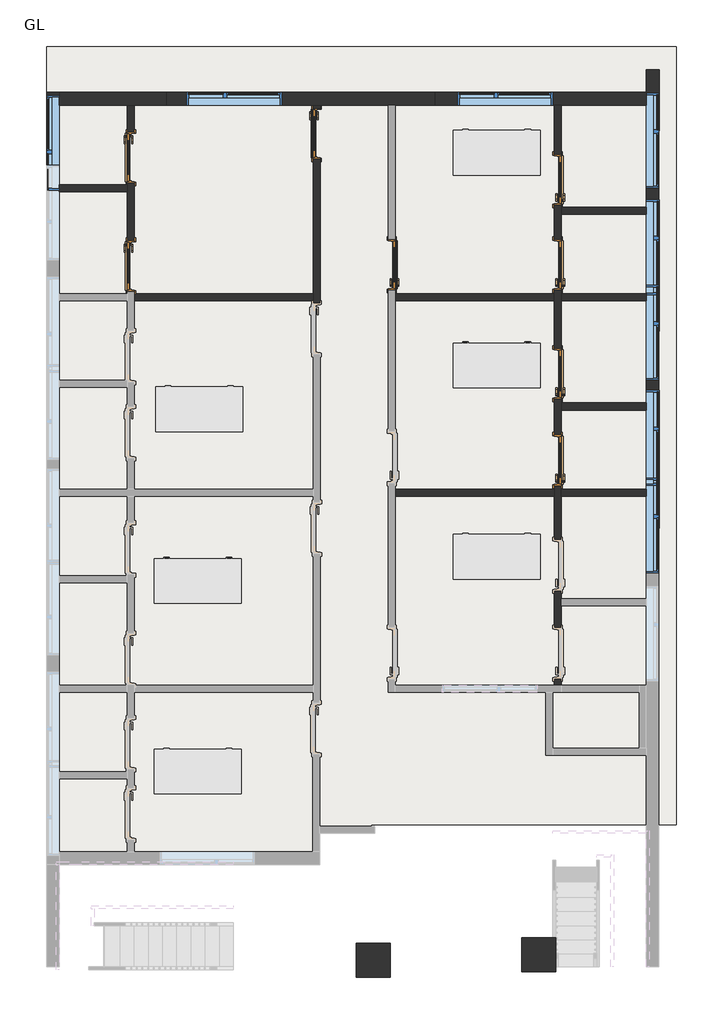
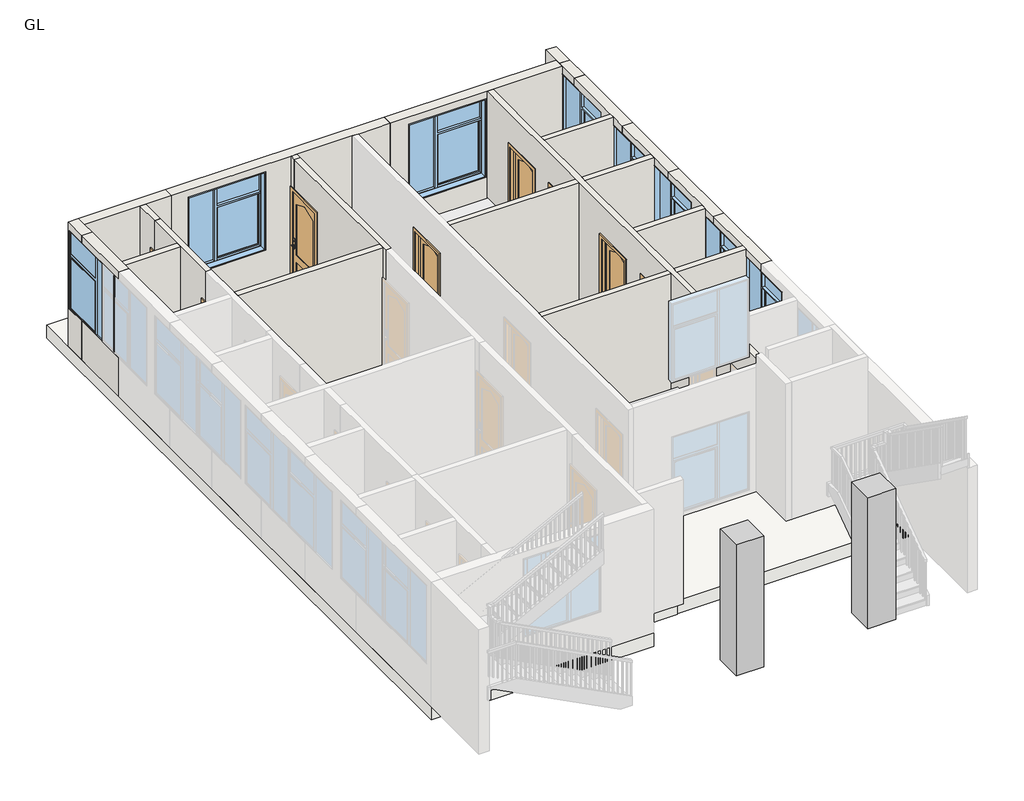
# One storey, part 2 of 4: 24 walls, 8 doors, 8 windows, 2 columns, 1 slab.
"""IFC4 building model written with IfcOpenShell, lengths in millimetres."""

from ifc_helpers import new_model, si_unit, frame, origin, origin_with_axes, place, context, project, spatial, polyline, outline, extrude, faceted_brep, transform, mapped, element, save
from components import column_c091e905, door_346b4a94, m_window_casement_double_sidelight_1702_x_1829mm_c8b42c7f

model = new_model("IFC4")

# Units and contexts
model_context = context("Model", 3, world=origin())
ifc_project = project(units=[si_unit("LENGTHUNIT", "METRE", prefix="MILLI")], contexts=[model_context])

# Site, building, storey
site = spatial("IfcSite", under=ifc_project)
building = spatial("IfcBuilding", under=site)
storey = spatial("IfcBuildingStorey", under=building, Name="GL", Elevation=0.0)

# Columns
placement = place(None, origin())
element("IfcColumn", 1, ObjectType="Rectangular Column : 24\" x 24\"", at=placement, inside=storey, context=model_context, shape_type="SweptSolid", body=[
    extrude(outline(polyline([(2657.4891134, -7132.8082131), (2657.4891134, -7742.4082131), (2047.8891134, -7742.4082131), (2047.8891134, -7132.8082131), (2657.4891134, -7132.8082131)])), origin_with_axes(), (0.0, 0.0, 1.0), 3048.0),
])
column_shape = column_c091e905(model_context)
element("IfcColumn", 2, ObjectType="Rectangular Column : 24\" x 24\"", at=placement, inside=storey, context=model_context, shape_type="MappedRepresentation", body=[
    mapped(column_shape, transform((-606.4108866, -7539.2082131, 0.0), x_axis=(1.0, 0.0, 0.0), y_axis=(0.0, 1.0, 0.0), z_axis=(0.0, 0.0, 1.0))),
])

# Doors
door_shape = door_346b4a94(model_context)
element("IfcDoor", 3, ObjectType="2'10\"X7'", at=placement, inside=storey, context=model_context, shape_type="MappedRepresentation", body=[
    mapped(door_shape, transform((2698.7641134, 6449.4399728, 0.0), x_axis=(0.0, -1.0, 0.0), y_axis=(1.0, 0.0, 0.0), z_axis=(0.0, 0.0, 1.0))),
])
element("IfcDoor", 4, ObjectType="2'10\"X7'", at=placement, inside=storey, context=model_context, shape_type="MappedRepresentation", body=[
    mapped(door_shape, transform((2698.7641134, 4925.4399728, 0.0), x_axis=(0.0, -1.0, 0.0), y_axis=(1.0, 0.0, 0.0), z_axis=(0.0, 0.0, 1.0))),
])
element("IfcDoor", 5, ObjectType="2'10\"X7'", at=placement, inside=storey, context=model_context, shape_type="MappedRepresentation", body=[
    mapped(door_shape, transform((2698.7641134, 2969.6399728, 0.0), x_axis=(0.0, -1.0, 0.0), y_axis=(1.0, 0.0, 0.0), z_axis=(0.0, 0.0, 1.0))),
])
element("IfcDoor", 6, ObjectType="2'10\"X7'", at=placement, inside=storey, context=model_context, shape_type="MappedRepresentation", body=[
    mapped(door_shape, transform((2698.7641134, 1420.2399728, 0.0), x_axis=(0.0, -1.0, 0.0), y_axis=(1.0, 0.0, 0.0), z_axis=(0.0, 0.0, 1.0))),
])
element("IfcDoor", 7, ObjectType="2'10\"X7'", at=placement, inside=storey, context=model_context, shape_type="MappedRepresentation", body=[
    mapped(door_shape, transform((-273.0358866, 4925.4399728, 0.0), x_axis=(0.0, -1.0, 0.0), y_axis=(1.0, 0.0, 0.0), z_axis=(0.0, 0.0, 1.0))),
])
element("IfcDoor", 8, ObjectType="2'10\"X7'", at=placement, inside=storey, context=model_context, shape_type="MappedRepresentation", body=[
    mapped(door_shape, transform((-4952.9858866, 4900.320652, 0.0), x_axis=(0.0, 1.0, 0.0), y_axis=(-1.0, 0.0, 0.0), z_axis=(0.0, 0.0, 1.0))),
])
element("IfcDoor", 9, ObjectType="2'10\"X7'", at=placement, inside=storey, context=model_context, shape_type="MappedRepresentation", body=[
    mapped(door_shape, transform((-4952.9858866, 6843.9929737, 0.0), x_axis=(0.0, 1.0, 0.0), y_axis=(-1.0, 0.0, 0.0), z_axis=(0.0, 0.0, 1.0))),
])
element("IfcDoor", 10, ObjectType="2'10\"X7'", at=placement, inside=storey, context=model_context, shape_type="MappedRepresentation", body=[
    mapped(door_shape, transform((-1625.5858866, 7274.3310623, 0.0), x_axis=(0.0, 1.0, 0.0), y_axis=(-1.0, 0.0, 0.0), z_axis=(0.0, 0.0, 1.0))),
])

# Slab
element("IfcSlab", 11, ObjectType="Generic - 12\"", at=placement, inside=storey, context=model_context, shape_type="SweptSolid", body=[
    extrude(outline(polyline([(4816.4891134, 8833.6177996), (4816.4891134, -5110.9822004), (-644.5108866, -5110.9822004), (-644.5108866, -5136.3822004), (-1562.4669858, -5136.3822004), (-1562.4669858, -5824.7082131), (-6461.1108866, -5824.7082131), (-6461.1108866, 8833.6177996), (4816.4891134, 8833.6177996)])), frame((0.0, 0.0, -304.8), z_axis=(0.0, 0.0, 1.0), x_axis=(1.0, 0.0, 0.0)), (0.0, 0.0, 1.0), 304.8),
])

# Walls
element("IfcWall", 12, ObjectType="Generic - 4.5\"", at=placement, inside=storey, context=model_context, shape_type="SweptSolid", body=[
    extrude(outline(polyline([(7782.9399728, 2895.6), (7782.9399728, 0.0), (7300.7929737, 0.0), (7300.7929737, 2158.6), (7224.9929737, 2158.6), (7224.9929737, 2895.6), (7782.9399728, 2895.6)])), frame((-5013.3108866, 0.0, 0.0), z_axis=(1.0, 0.0, 0.0), x_axis=(0.0, 1.0, 0.0)), (0.0, 0.0, 1.0), 127.0),
])
element("IfcWall", 13, ObjectType="Generic - 4.5\"", at=placement, inside=storey, context=model_context, shape_type="Brep", body=[
    faceted_brep([(-5013.3108866, 5281.320652, 2158.6), (-5013.3108866, 5281.320652, 2895.6), (-5013.3108866, 6233.5399728, 2895.6), (-5013.3108866, 6360.5399728, 2895.6), (-5013.3108866, 7224.9929737, 2895.6), (-5013.3108866, 7224.9929737, 2158.6), (-5013.3108866, 6387.1929737, 2158.6), (-5013.3108866, 6387.1929737, 0.0), (-5013.3108866, 6360.5399728, 0.0), (-5013.3108866, 6233.5399728, 0.0), (-5013.3108866, 5357.120652, 0.0), (-5013.3108866, 5357.120652, 2158.6), (-4886.3108866, 5281.320652, 2895.6), (-4886.3108866, 5281.320652, 2158.6), (-4886.3108866, 5357.120652, 2158.6), (-4886.3108866, 5357.120652, 0.0), (-4886.3108866, 6387.1929737, 0.0), (-4886.3108866, 6387.1929737, 2158.6), (-4886.3108866, 7224.9929737, 2158.6), (-4886.3108866, 7224.9929737, 2895.6)], [[[0, 1, 2, 3, 4, 5, 6, 7, 8, 9, 10, 11]], [[12, 13, 14, 15, 16, 17, 18, 19]], [[15, 10, 9, 8, 7, 16]], [[1, 0, 13, 12]], [[4, 19, 18, 5]], [[14, 11, 10, 15]], [[11, 14, 13, 0]], [[17, 6, 5, 18]], [[6, 17, 16, 7]], [[4, 3, 2, 1, 12, 19]]]),
])
element("IfcWall", 14, ObjectType="Generic - 4.5\"", at=placement, inside=storey, context=model_context, shape_type="SweptSolid", body=[
    extrude(outline(polyline([(-5013.3108866, 6233.5399728), (-6232.5508078, 6233.5399728), (-6232.5508078, 6360.5399728), (-5013.3108866, 6360.5399728), (-5013.3108866, 6233.5399728)])), origin_with_axes(), (0.0, 0.0, 1.0), 2895.6),
])
element("IfcWall", 15, ObjectType="Generic - 4.5\"", at=placement, inside=storey, context=model_context, shape_type="SweptSolid", body=[
    extrude(outline(polyline([(-1685.9108866, 4277.7399728), (-4886.3108866, 4277.7399728), (-4886.3108866, 4404.7399728), (-1685.9108866, 4404.7399728), (-1685.9108866, 4277.7399728)])), origin_with_axes(), (0.0, 0.0, 1.0), 2895.6),
])
element("IfcWall", 16, ObjectType="Generic - 4.5\"", at=placement, inside=storey, context=model_context, shape_type="SweptSolid", body=[
    extrude(outline(polyline([(7782.9399728, 2895.6), (7782.9399728, 0.0), (7731.1310623, 0.0), (7731.1310623, 2158.6), (7655.3310623, 2158.6), (7655.3310623, 2895.6), (7782.9399728, 2895.6)])), frame((-1685.9108866, 0.0, 0.0), z_axis=(1.0, 0.0, 0.0), x_axis=(0.0, 1.0, 0.0)), (0.0, 0.0, 1.0), 127.0),
])
element("IfcWall", 17, ObjectType="Generic - 4.5\"", at=placement, inside=storey, context=model_context, shape_type="Brep", body=[
    faceted_brep([(-1685.9108866, 4182.2008884, 2158.6), (-1685.9108866, 4182.2008884, 2895.6), (-1685.9108866, 4277.7399728, 2895.6), (-1685.9108866, 4404.7399728, 2895.6), (-1685.9108866, 7655.3310623, 2895.6), (-1685.9108866, 7655.3310623, 2158.6), (-1685.9108866, 6817.5310623, 2158.6), (-1685.9108866, 6817.5310623, 0.0), (-1685.9108866, 4404.7399728, 0.0), (-1685.9108866, 4277.7399728, 0.0), (-1685.9108866, 4232.6008884, 0.0), (-1685.9108866, 4232.6008884, 2158.6), (-1558.9108866, 4182.2008884, 2895.6), (-1558.9108866, 4182.2008884, 2158.6), (-1558.9108866, 4232.6008884, 2158.6), (-1558.9108866, 4232.6008884, 0.0), (-1558.9108866, 6817.5310623, 0.0), (-1558.9108866, 6817.5310623, 2158.6), (-1558.9108866, 7655.3310623, 2158.6), (-1558.9108866, 7655.3310623, 2895.6), (-1685.4871817, 4182.2008884, 2158.6), (-1685.4871817, 4182.2008884, 2895.6)], [[[0, 1, 2, 3, 4, 5, 6, 7, 8, 9, 10, 11]], [[12, 13, 14, 15, 16, 17, 18, 19]], [[15, 10, 9, 8, 7, 16]], [[1, 0, 20, 13, 12, 21]], [[4, 19, 18, 5]], [[14, 11, 10, 15]], [[11, 14, 13, 20, 0]], [[17, 6, 5, 18]], [[6, 17, 16, 7]], [[4, 3, 2, 1, 21, 12, 19]]]),
])
element("IfcWall", 18, ObjectType="Generic - 4.5\"", at=placement, inside=storey, context=model_context, shape_type="Brep", body=[
    faceted_brep([(2632.0891134, 7782.9399728, 2895.6), (2632.0891134, 7782.9399728, 0.0), (2632.0891134, 6906.2399728, 0.0), (2632.0891134, 6906.2399728, 2158.6), (2632.0891134, 5992.6399728, 2158.6), (2632.0891134, 5992.6399728, 0.0), (2632.0891134, 5382.2399728, 0.0), (2632.0891134, 5382.2399728, 2158.6), (2632.0891134, 4468.6399728, 2158.6), (2632.0891134, 4468.6399728, 0.0), (2632.0891134, 4404.7399728, 0.0), (2632.0891134, 4277.7399728, 0.0), (2632.0891134, 3426.4399728, 0.0), (2632.0891134, 3426.4399728, 2158.6), (2632.0891134, 2512.8399728, 2158.6), (2632.0891134, 2512.8399728, 0.0), (2632.0891134, 1877.0399728, 0.0), (2632.0891134, 1877.0399728, 2158.6), (2632.0891134, 963.4399728, 2158.6), (2632.0891134, 963.4399728, 0.0), (2632.0891134, 899.5399728, 0.0), (2632.0891134, 772.5399728, 0.0), (2632.0891134, -2.5600272, 0.0), (2632.0891134, -2.5600272, 2158.6), (2632.0891134, -916.1600272, 2158.6), (2632.0891134, -916.1600272, 0.0), (2632.0891134, -1577.3600272, 0.0), (2632.0891134, -1577.3600272, 2158.6), (2632.0891134, -2490.9600272, 2158.6), (2632.0891134, -2490.9600272, 0.0), (2632.0891134, -2605.6600272, 0.0), (2632.0891134, -2605.6600272, 2895.6), (2632.0891134, 772.5399728, 2895.6), (2632.0891134, 899.5399728, 2895.6), (2632.0891134, 4277.7399728, 2895.6), (2632.0891134, 4404.7399728, 2895.6), (2759.0891134, 7782.9399728, 0.0), (2759.0891134, 7782.9399728, 2895.6), (2759.0891134, 5954.1399728, 2895.6), (2759.0891134, 5827.1399728, 2895.6), (2759.0891134, 4404.7399728, 2895.6), (2759.0891134, 4277.7399728, 2895.6), (2759.0891134, 2448.9399728, 2895.6), (2759.0891134, 2321.9399728, 2895.6), (2759.0891134, 899.5399728, 2895.6), (2759.0891134, 772.5399728, 2895.6), (2759.0891134, -1056.2600272, 2895.6), (2759.0891134, -1183.2600272, 2895.6), (2759.0891134, -2605.6600272, 2895.6), (2759.0891134, -2605.6600272, 0.0), (2759.0891134, -2490.9600272, 0.0), (2759.0891134, -2490.9600272, 2158.6), (2759.0891134, -1577.3600272, 2158.6), (2759.0891134, -1577.3600272, 0.0), (2759.0891134, -1183.2600272, 0.0), (2759.0891134, -1056.2600272, 0.0), (2759.0891134, -916.1600272, 0.0), (2759.0891134, -916.1600272, 2158.6), (2759.0891134, -2.5600272, 2158.6), (2759.0891134, -2.5600272, 0.0), (2759.0891134, 772.5399728, 0.0), (2759.0891134, 899.5399728, 0.0), (2759.0891134, 963.4399728, 0.0), (2759.0891134, 963.4399728, 2158.6), (2759.0891134, 1877.0399728, 2158.6), (2759.0891134, 1877.0399728, 0.0), (2759.0891134, 2321.9399728, 0.0), (2759.0891134, 2448.9399728, 0.0), (2759.0891134, 2512.8399728, 0.0), (2759.0891134, 2512.8399728, 2158.6), (2759.0891134, 3426.4399728, 2158.6), (2759.0891134, 3426.4399728, 0.0), (2759.0891134, 4277.7399728, 0.0), (2759.0891134, 4404.7399728, 0.0), (2759.0891134, 4468.6399728, 0.0), (2759.0891134, 4468.6399728, 2158.6), (2759.0891134, 5382.2399728, 2158.6), (2759.0891134, 5382.2399728, 0.0), (2759.0891134, 5827.1399728, 0.0), (2759.0891134, 5954.1399728, 0.0), (2759.0891134, 5992.6399728, 0.0), (2759.0891134, 5992.6399728, 2158.6), (2759.0891134, 6906.2399728, 2158.6), (2759.0891134, 6906.2399728, 0.0)], [[[0, 1, 2, 3, 4, 5, 6, 7, 8, 9, 10, 11, 12, 13, 14, 15, 16, 17, 18, 19, 20, 21, 22, 23, 24, 25, 26, 27, 28, 29, 30, 31, 32, 33, 34, 35]], [[36, 37, 38, 39, 40, 41, 42, 43, 44, 45, 46, 47, 48, 49, 50, 51, 52, 53, 54, 55, 56, 57, 58, 59, 60, 61, 62, 63, 64, 65, 66, 67, 68, 69, 70, 71, 72, 73, 74, 75, 76, 77, 78, 79, 80, 81, 82, 83]], [[1, 36, 83, 2]], [[5, 80, 79, 78, 77, 6]], [[9, 74, 73, 72, 71, 12, 11, 10]], [[15, 68, 67, 66, 65, 16]], [[19, 62, 61, 60, 59, 22, 21, 20]], [[25, 56, 55, 54, 53, 26]], [[49, 30, 29, 50]], [[1, 0, 37, 36]], [[4, 81, 80, 5]], [[81, 4, 3, 82]], [[82, 3, 2, 83]], [[9, 8, 75, 74]], [[8, 7, 76, 75]], [[7, 6, 77, 76]], [[14, 69, 68, 15]], [[69, 14, 13, 70]], [[70, 13, 12, 71]], [[18, 63, 62, 19]], [[63, 18, 17, 64]], [[64, 17, 16, 65]], [[24, 57, 56, 25]], [[57, 24, 23, 58]], [[58, 23, 22, 59]], [[28, 51, 50, 29]], [[51, 28, 27, 52]], [[52, 27, 26, 53]], [[0, 35, 34, 33, 32, 31, 48, 47, 46, 45, 44, 43, 42, 41, 40, 39, 38, 37]], [[31, 30, 49, 48]]]),
])
element("IfcWall", 19, ObjectType="Generic - 4.5\"", at=placement, inside=storey, context=model_context, shape_type="SweptSolid", body=[
    extrude(outline(polyline([(2632.0891134, 4277.7399728), (-212.7108866, 4277.7399728), (-212.7108866, 4404.7399728), (2632.0891134, 4404.7399728), (2632.0891134, 4277.7399728)])), origin_with_axes(), (0.0, 0.0, 1.0), 2895.6),
])
element("IfcWall", 20, ObjectType="Generic - 4.5\"", at=placement, inside=storey, context=model_context, shape_type="SweptSolid", body=[
    extrude(outline(polyline([(2632.0891134, 772.5399728), (-212.7108866, 772.5399728), (-212.7108866, 899.5399728), (2632.0891134, 899.5399728), (2632.0891134, 772.5399728)])), origin_with_axes(), (0.0, 0.0, 1.0), 2895.6),
])
element("IfcWall", 21, ObjectType="Generic - 4.5\"", at=placement, inside=storey, context=model_context, shape_type="SweptSolid", body=[
    extrude(outline(polyline([(4281.587404, 5827.1399728), (2759.0891134, 5827.1399728), (2759.0891134, 5954.1399728), (4281.587404, 5954.1399728), (4281.587404, 5827.1399728)])), origin_with_axes(), (0.0, 0.0, 1.0), 2895.6),
])
element("IfcWall", 22, ObjectType="Generic - 4.5\"", at=placement, inside=storey, context=model_context, shape_type="SweptSolid", body=[
    extrude(outline(polyline([(4283.9989713, 4277.7399728), (2759.0891134, 4277.7399728), (2759.0891134, 4404.7399728), (4283.9989713, 4404.7399728), (4283.9989713, 4277.7399728)])), origin_with_axes(), (0.0, 0.0, 1.0), 2895.6),
])
element("IfcWall", 23, ObjectType="Generic - 4.5\"", at=placement, inside=storey, context=model_context, shape_type="SweptSolid", body=[
    extrude(outline(polyline([(4281.0767915, 2321.9399728), (2759.0891134, 2321.9399728), (2759.0891134, 2448.9399728), (4281.0767915, 2448.9399728), (4281.0767915, 2321.9399728)])), origin_with_axes(), (0.0, 0.0, 1.0), 2895.6),
])
element("IfcWall", 24, ObjectType="Generic - 4.5\"", at=placement, inside=storey, context=model_context, shape_type="SweptSolid", body=[
    extrude(outline(polyline([(4283.0918814, 772.5399728), (2759.0891134, 772.5399728), (2759.0891134, 899.5399728), (4283.0918814, 899.5399728), (4283.0918814, 772.5399728)])), origin_with_axes(), (0.0, 0.0, 1.0), 2895.6),
])
element("IfcWall", 25, ObjectType="Generic - 9\"", at=placement, inside=storey, context=model_context, shape_type="Brep", body=[
    faceted_brep([(-6232.5108866, 7782.9399728, 0.0), (-5013.3108866, 7782.9399728, 0.0), (-4886.3108866, 7782.9399728, 0.0), (-4318.2603585, 7782.9399728, 0.0), (-4318.2603585, 7782.9399728, 2895.6), (-4886.3108866, 7782.9399728, 2895.6), (-5013.3108866, 7782.9399728, 2895.6), (-6232.5108866, 7782.9399728, 2895.6), (-6232.5108866, 8011.5399728, 0.0), (-6232.5108866, 8011.5399728, 2895.6), (-4318.2603585, 8011.5399728, 2895.6), (-4318.2603585, 8011.5399728, 0.0)], [[[0, 1, 2, 3, 4, 5, 6, 7]], [[8, 9, 10, 11]], [[3, 2, 1, 0, 8, 11]], [[4, 3, 11, 10]], [[0, 7, 9, 8]], [[7, 6, 5, 4, 10, 9]]]),
])
element("IfcWall", 26, ObjectType="Generic - 9\"", at=placement, inside=storey, context=model_context, shape_type="Brep", body=[
    faceted_brep([(-4318.2603585, 7782.9399728, 0.0), (-1685.9108866, 7782.9399728, 0.0), (-1558.9108866, 7782.9399728, 0.0), (-339.7108866, 7782.9399728, 0.0), (-212.7108866, 7782.9399728, 0.0), (496.3553976, 7782.9399728, 0.0), (496.3553976, 7782.9399728, 2895.6), (-212.7108866, 7782.9399728, 2895.6), (-339.7108866, 7782.9399728, 2895.6), (-1558.9108866, 7782.9399728, 2895.6), (-1685.9108866, 7782.9399728, 2895.6), (-4318.2603585, 7782.9399728, 2895.6), (-2248.1603585, 7782.9399728, 2728.8), (-2248.1603585, 7782.9399728, 900.0), (-3949.9603585, 7782.9399728, 900.0), (-3949.9603585, 7782.9399728, 2728.8), (-4318.2603585, 8011.5399728, 0.0), (-4318.2603585, 8011.5399728, 2895.6), (496.3553976, 8011.5399728, 2895.6), (496.3553976, 8011.5399728, 0.0), (-2248.1603585, 8011.5399728, 2728.8), (-3949.9603585, 8011.5399728, 2728.8), (-3949.9603585, 8011.5399728, 900.0), (-2248.1603585, 8011.5399728, 900.0)], [[[0, 1, 2, 3, 4, 5, 6, 7, 8, 9, 10, 11], [12, 13, 14, 15]], [[16, 17, 18, 19], [20, 21, 22, 23]], [[5, 4, 3, 2, 1, 0, 16, 19]], [[6, 5, 19, 18]], [[0, 11, 17, 16]], [[13, 12, 20, 23]], [[14, 13, 23, 22]], [[15, 14, 22, 21]], [[12, 15, 21, 20]], [[11, 10, 9, 8, 7, 6, 18, 17]]]),
])
element("IfcWall", 27, ObjectType="Generic - 9\"", at=placement, inside=storey, context=model_context, shape_type="Brep", body=[
    faceted_brep([(496.3553976, 7782.9399728, 0.0), (2632.0891134, 7782.9399728, 0.0), (2759.0891134, 7782.9399728, 0.0), (4283.0891134, 7782.9399728, 0.0), (4283.0891134, 7782.9399728, 2895.6), (2759.0891134, 7782.9399728, 2895.6), (2632.0891134, 7782.9399728, 2895.6), (496.3553976, 7782.9399728, 2895.6), (2606.6891134, 7782.9399728, 2728.8), (2606.6891134, 7782.9399728, 900.0), (904.8891134, 7782.9399728, 900.0), (904.8891134, 7782.9399728, 2728.8), (496.3553976, 8011.5399728, 0.0), (496.3553976, 8011.5399728, 2895.6), (4283.0891134, 8011.5399728, 2895.6), (4283.0891134, 8011.5399728, 0.0), (2606.6891134, 8011.5399728, 2728.8), (904.8891134, 8011.5399728, 2728.8), (904.8891134, 8011.5399728, 900.0), (2606.6891134, 8011.5399728, 900.0), (4283.0891134, 7897.2399728, 0.0), (4283.0891134, 7897.2399728, 2895.6)], [[[0, 1, 2, 3, 4, 5, 6, 7], [8, 9, 10, 11]], [[12, 13, 14, 15], [16, 17, 18, 19]], [[3, 2, 1, 0, 12, 15, 20]], [[0, 7, 13, 12]], [[9, 8, 16, 19]], [[10, 9, 19, 18]], [[11, 10, 18, 17]], [[8, 11, 17, 16]], [[4, 3, 20, 15, 14, 21]], [[7, 6, 5, 4, 21, 14, 13]]]),
])
element("IfcWall", 28, ObjectType="Generic - 9\"", at=placement, inside=storey, context=model_context, shape_type="Brep", body=[
    faceted_brep([(4283.0891134, 7897.2399728, 0.0), (4283.0891134, 7782.9399728, 0.0), (4283.0891134, 7325.7399728, 0.0), (4283.0891134, 7325.7399728, 900.0), (4283.0891134, 7897.2399728, 900.0), (4511.6891134, 7325.7399728, 0.0), (4511.6891134, 7897.2399728, 0.0), (4511.6891134, 7897.2399728, 900.0), (4511.6891134, 7325.7399728, 900.0), (4510.187404, 7325.7399728, 0.0), (4510.187404, 7325.7399728, 900.0)], [[[0, 1, 2, 3, 4]], [[5, 6, 7, 8]], [[2, 1, 0, 6, 5, 9]], [[2, 9, 5, 8, 10, 3]], [[6, 0, 4, 7]], [[4, 3, 10, 8, 7]]]),
    faceted_brep([(4283.0891134, 7325.7399728, 2895.6), (4283.0891134, 7782.9399728, 2895.6), (4283.0891134, 7897.2399728, 2895.6), (4283.0891134, 7897.2399728, 2728.8), (4283.0891134, 7325.7399728, 2728.8), (4511.6891134, 7897.2399728, 2895.6), (4511.6891134, 7325.7399728, 2895.6), (4511.6891134, 7325.7399728, 2728.8), (4511.6891134, 7897.2399728, 2728.8), (4510.187404, 7325.7399728, 2895.6), (4510.187404, 7325.7399728, 2728.8)], [[[0, 1, 2, 3, 4]], [[5, 6, 7, 8]], [[6, 9, 0, 4, 10, 7]], [[2, 5, 8, 3]], [[4, 3, 8, 7, 10]], [[2, 1, 0, 9, 6, 5]]]),
])
element("IfcWall", 29, ObjectType="Generic - 9\"", at=placement, inside=storey, context=model_context, shape_type="Brep", body=[
    faceted_brep([(4281.587404, 7325.7399728, 0.0), (4281.587404, 5954.1399728, 0.0), (4281.587404, 5827.1399728, 0.0), (4281.587404, 5490.9915892, 0.0), (4281.587404, 5490.9915892, 900.0), (4281.587404, 6087.8915892, 900.0), (4281.587404, 6087.8915892, 2728.8), (4281.587404, 5490.9915892, 2728.8), (4281.587404, 5490.9915892, 2895.6), (4281.587404, 5827.1399728, 2895.6), (4281.587404, 5954.1399728, 2895.6), (4281.587404, 7325.7399728, 2895.6), (4281.587404, 7325.7399728, 2728.8), (4281.587404, 6297.0399728, 2728.8), (4281.587404, 6297.0399728, 900.0), (4281.587404, 7325.7399728, 900.0), (4510.187404, 5490.9915892, 0.0), (4510.187404, 7325.7399728, 0.0), (4510.187404, 7325.7399728, 900.0), (4510.187404, 6297.0399728, 900.0), (4510.187404, 6297.0399728, 2728.8), (4510.187404, 7325.7399728, 2728.8), (4510.187404, 7325.7399728, 2895.6), (4510.187404, 5490.9915892, 2895.6), (4510.187404, 5490.9915892, 2728.8), (4510.187404, 6087.8915892, 2728.8), (4510.187404, 6087.8915892, 900.0), (4510.187404, 5490.9915892, 900.0), (4283.0891134, 7325.7399728, 0.0), (4283.9989713, 5490.9915892, 0.0), (4283.9989713, 5490.9915892, 900.0), (4283.9989713, 5490.9915892, 2895.6), (4283.9989713, 5490.9915892, 2728.8), (4283.0891134, 7325.7399728, 900.0), (4283.0891134, 7325.7399728, 2895.6), (4283.0891134, 7325.7399728, 2728.8)], [[[0, 1, 2, 3, 4, 5, 6, 7, 8, 9, 10, 11, 12, 13, 14, 15]], [[16, 17, 18, 19, 20, 21, 22, 23, 24, 25, 26, 27]], [[3, 2, 1, 0, 28, 17, 16, 29]], [[3, 29, 16, 27, 30, 4]], [[23, 31, 8, 7, 32, 24]], [[17, 28, 0, 15, 33, 18]], [[12, 11, 34, 22, 21, 35]], [[13, 20, 19, 14]], [[14, 19, 18, 33, 15]], [[20, 13, 12, 35, 21]], [[26, 5, 4, 30, 27]], [[5, 26, 25, 6]], [[6, 25, 24, 32, 7]], [[11, 10, 9, 8, 31, 23, 22, 34]]]),
])
element("IfcWall", 30, ObjectType="Generic - 9\"", at=placement, inside=storey, context=model_context, shape_type="Brep", body=[
    faceted_brep([(4283.9989713, 5490.9915892, 0.0), (4283.9989713, 4404.7399728, 0.0), (4283.9989713, 4277.7399728, 0.0), (4283.9989713, 3730.8359967, 0.0), (4283.9989713, 3730.8359967, 900.0), (4283.9989713, 5490.9915892, 900.0), (4512.5989713, 3730.8359967, 0.0), (4512.5989713, 5490.9915892, 0.0), (4512.5989713, 5490.9915892, 900.0), (4512.5989713, 3730.8359967, 900.0), (4510.187404, 5490.9915892, 0.0), (4509.6767915, 3730.8359967, 0.0), (4509.6767915, 3730.8359967, 900.0), (4510.187404, 5490.9915892, 900.0)], [[[0, 1, 2, 3, 4, 5]], [[6, 7, 8, 9]], [[3, 2, 1, 0, 10, 7, 6, 11]], [[3, 11, 6, 9, 12, 4]], [[7, 10, 0, 5, 13, 8]], [[8, 13, 5, 4, 12, 9]]]),
    faceted_brep([(4283.9989713, 5490.9915892, 2895.6), (4283.9989713, 5490.9915892, 2728.8), (4283.9989713, 3730.8359967, 2728.8), (4283.9989713, 3730.8359967, 2895.6), (4283.9989713, 4277.7399728, 2895.6), (4283.9989713, 4404.7399728, 2895.6), (4512.5989713, 3730.8359967, 2728.8), (4512.5989713, 5490.9915892, 2728.8), (4512.5989713, 5490.9915892, 2895.6), (4512.5989713, 3730.8359967, 2895.6), (4509.6767915, 3730.8359967, 2895.6), (4509.6767915, 3730.8359967, 2728.8), (4510.187404, 5490.9915892, 2895.6), (4510.187404, 5490.9915892, 2728.8)], [[[0, 1, 2, 3, 4, 5]], [[6, 7, 8, 9]], [[9, 10, 3, 2, 11, 6]], [[1, 0, 12, 8, 7, 13]], [[1, 13, 7, 6, 11, 2]], [[0, 5, 4, 3, 10, 9, 8, 12]]]),
])
element("IfcWall", 31, ObjectType="Generic - 9\"", at=placement, inside=storey, context=model_context, shape_type="Brep", body=[
    faceted_brep([(4281.0767915, 3730.8359967, 0.0), (4281.0767915, 2448.9399728, 0.0), (4281.0767915, 2321.9399728, 0.0), (4281.0767915, 2023.9001312, 0.0), (4281.0767915, 2023.9001312, 900.0), (4281.0767915, 2671.6001312, 900.0), (4281.0767915, 2671.6001312, 2728.8), (4281.0767915, 2023.9001312, 2728.8), (4281.0767915, 2023.9001312, 2895.6), (4281.0767915, 2321.9399728, 2895.6), (4281.0767915, 2448.9399728, 2895.6), (4281.0767915, 3730.8359967, 2895.6), (4281.0767915, 3730.8359967, 2728.8), (4281.0767915, 2854.5359967, 2728.8), (4281.0767915, 2854.5359967, 900.0), (4281.0767915, 3730.8359967, 900.0), (4509.6767915, 2023.9001312, 0.0), (4509.6767915, 3730.8359967, 0.0), (4509.6767915, 3730.8359967, 900.0), (4509.6767915, 2854.5359967, 900.0), (4509.6767915, 2854.5359967, 2728.8), (4509.6767915, 3730.8359967, 2728.8), (4509.6767915, 3730.8359967, 2895.6), (4509.6767915, 2023.9001312, 2895.6), (4509.6767915, 2023.9001312, 2728.8), (4509.6767915, 2671.6001312, 2728.8), (4509.6767915, 2671.6001312, 900.0), (4509.6767915, 2023.9001312, 900.0), (4283.9989713, 3730.8359967, 0.0), (4283.0918814, 2023.9001312, 0.0), (4283.0918814, 2023.9001312, 900.0), (4283.0918814, 2023.9001312, 2895.6), (4283.0918814, 2023.9001312, 2728.8), (4283.9989713, 3730.8359967, 900.0), (4283.9989713, 3730.8359967, 2895.6), (4283.9989713, 3730.8359967, 2728.8)], [[[0, 1, 2, 3, 4, 5, 6, 7, 8, 9, 10, 11, 12, 13, 14, 15]], [[16, 17, 18, 19, 20, 21, 22, 23, 24, 25, 26, 27]], [[3, 2, 1, 0, 28, 17, 16, 29]], [[3, 29, 16, 27, 30, 4]], [[23, 31, 8, 7, 32, 24]], [[17, 28, 0, 15, 33, 18]], [[12, 11, 34, 22, 21, 35]], [[13, 20, 19, 14]], [[14, 19, 18, 33, 15]], [[20, 13, 12, 35, 21]], [[26, 5, 4, 30, 27]], [[5, 26, 25, 6]], [[6, 25, 24, 32, 7]], [[11, 10, 9, 8, 31, 23, 22, 34]]]),
])
element("IfcWall", 32, ObjectType="Generic - 9\"", at=placement, inside=storey, context=model_context, shape_type="Brep", body=[
    faceted_brep([(4283.0918814, 2023.9001312, 0.0), (4283.0918814, 899.5399728, 0.0), (4283.0918814, 772.5399728, 0.0), (4283.0918814, 200.5184135, 0.0), (4283.0918814, 200.5184135, 900.0), (4283.0918814, 2023.9001312, 900.0), (4511.6918814, 200.5184135, 0.0), (4511.6918814, 2023.9001312, 0.0), (4511.6918814, 2023.9001312, 900.0), (4511.6918814, 200.5184135, 900.0), (4509.6767915, 2023.9001312, 0.0), (4510.3311655, 200.5184135, 0.0), (4510.3311655, 200.5184135, 900.0), (4509.6767915, 2023.9001312, 900.0)], [[[0, 1, 2, 3, 4, 5]], [[6, 7, 8, 9]], [[3, 2, 1, 0, 10, 7, 6, 11]], [[3, 11, 6, 9, 12, 4]], [[7, 10, 0, 5, 13, 8]], [[8, 13, 5, 4, 12, 9]]]),
    faceted_brep([(4283.0918814, 2023.9001312, 2895.6), (4283.0918814, 2023.9001312, 2728.8), (4283.0918814, 200.5184135, 2728.8), (4283.0918814, 200.5184135, 2895.6), (4283.0918814, 772.5399728, 2895.6), (4283.0918814, 899.5399728, 2895.6), (4511.6918814, 200.5184135, 2728.8), (4511.6918814, 2023.9001312, 2728.8), (4511.6918814, 2023.9001312, 2895.6), (4511.6918814, 200.5184135, 2895.6), (4510.3311655, 200.5184135, 2895.6), (4510.3311655, 200.5184135, 2728.8), (4509.6767915, 2023.9001312, 2895.6), (4509.6767915, 2023.9001312, 2728.8)], [[[0, 1, 2, 3, 4, 5]], [[6, 7, 8, 9]], [[9, 10, 3, 2, 11, 6]], [[1, 0, 12, 8, 7, 13]], [[1, 13, 7, 6, 11, 2]], [[0, 5, 4, 3, 10, 9, 8, 12]]]),
])
element("IfcWall", 33, ObjectType="Generic - 9\"", at=placement, inside=storey, context=model_context, shape_type="Brep", body=[
    faceted_brep([(-6232.5508078, 6088.0863192, 0.0), (-6232.5508078, 6233.5399728, 0.0), (-6232.5508078, 6360.5399728, 0.0), (-6232.5508078, 7490.3748838, 0.0), (-6232.5508078, 7490.3748838, 900.0), (-6232.5508078, 6088.0863192, 900.0), (-6461.1508078, 7490.3748838, 0.0), (-6461.1508078, 6088.0863192, 0.0), (-6461.1508078, 6088.0863192, 900.0), (-6461.1508078, 7490.3748838, 900.0)], [[[0, 1, 2, 3, 4, 5]], [[6, 7, 8, 9]], [[3, 2, 1, 0, 7, 6]], [[3, 6, 9, 4]], [[7, 0, 5, 8]], [[4, 9, 8, 5]]]),
    faceted_brep([(-6232.5508078, 6088.0863192, 2728.8), (-6232.5508078, 7490.3748838, 2728.8), (-6232.5508078, 7490.3748838, 2895.6), (-6232.5508078, 6360.5399728, 2895.6), (-6232.5508078, 6233.5399728, 2895.6), (-6232.5508078, 6088.0863192, 2895.6), (-6461.1508078, 7490.3748838, 2895.6), (-6461.1508078, 7490.3748838, 2728.8), (-6461.1508078, 6088.0863192, 2728.8), (-6461.1508078, 6088.0863192, 2895.6)], [[[0, 1, 2, 3, 4, 5]], [[6, 7, 8, 9]], [[2, 1, 7, 6]], [[5, 9, 8, 0]], [[7, 1, 0, 8]], [[5, 4, 3, 2, 6, 9]]]),
])
element("IfcWall", 34, ObjectType="Generic - 9\"", at=placement, inside=storey, context=model_context, shape_type="Brep", body=[
    faceted_brep([(-6232.5108866, 7490.3748838, 0.0), (-6232.5108866, 7782.9399728, 0.0), (-6232.5108866, 8011.5399728, 0.0), (-6232.5108866, 8011.5399728, 2895.6), (-6232.5108866, 7782.9399728, 2895.6), (-6232.5108866, 7490.3748838, 2895.6), (-6232.5108866, 7490.3748838, 2728.8), (-6232.5108866, 7960.2748838, 2728.8), (-6232.5108866, 7960.2748838, 900.0), (-6232.5108866, 7490.3748838, 900.0), (-6461.1108866, 8011.5399728, 0.0), (-6461.1108866, 7490.3748838, 0.0), (-6461.1108866, 7490.3748838, 900.0), (-6461.1108866, 7960.2748838, 900.0), (-6461.1108866, 7960.2748838, 2728.8), (-6461.1108866, 7490.3748838, 2728.8), (-6461.1108866, 7490.3748838, 2895.6), (-6461.1108866, 8011.5399728, 2895.6)], [[[0, 1, 2, 3, 4, 5, 6, 7, 8, 9]], [[10, 11, 12, 13, 14, 15, 16, 17]], [[2, 1, 0, 11, 10]], [[11, 0, 9, 12]], [[5, 16, 15, 6]], [[7, 14, 13, 8]], [[8, 13, 12, 9]], [[14, 7, 6, 15]], [[3, 2, 10, 17]], [[5, 4, 3, 17, 16]]]),
])
element("IfcWall", 35, ObjectType="Generic - 9\"", at=placement, inside=storey, context=model_context, shape_type="Brep", body=[
    faceted_brep([(4283.0891134, 8414.5177996, 0.0), (4283.0891134, 8011.5399728, 0.0), (4283.0891134, 7897.2399728, 0.0), (4283.0891134, 7897.2399728, 900.0), (4283.0891134, 7998.8399728, 900.0), (4283.0891134, 7998.8399728, 2728.8), (4283.0891134, 7897.2399728, 2728.8), (4283.0891134, 7897.2399728, 2895.6), (4283.0891134, 8011.5399728, 2895.6), (4283.0891134, 8414.5177996, 2895.6), (4511.6891134, 7897.2399728, 0.0), (4511.6891134, 8414.5177996, 0.0), (4511.6891134, 8414.5177996, 2895.6), (4511.6891134, 7897.2399728, 2895.6), (4511.6891134, 7897.2399728, 2728.8), (4511.6891134, 7998.8399728, 2728.8), (4511.6891134, 7998.8399728, 900.0), (4511.6891134, 7897.2399728, 900.0)], [[[0, 1, 2, 3, 4, 5, 6, 7, 8, 9]], [[10, 11, 12, 13, 14, 15, 16, 17]], [[2, 1, 0, 11, 10]], [[2, 10, 17, 3]], [[13, 7, 6, 14]], [[0, 9, 12, 11]], [[16, 4, 3, 17]], [[4, 16, 15, 5]], [[5, 15, 14, 6]], [[9, 8, 7, 13, 12]]]),
])

# Windows
m_window_casement_double_sidelight_1702_x_1829mm_shape = m_window_casement_double_sidelight_1702_x_1829mm_c8b42c7f(model_context)
element("IfcWindow", 36, ObjectType="M_Window-Casement-Double-Sidelight : 1702 x 1829mm", at=placement, inside=storey, context=model_context, shape_type="MappedRepresentation", body=[
    mapped(m_window_casement_double_sidelight_1702_x_1829mm_shape, transform((-6346.8508078, 7109.3748838, 0.0), x_axis=(0.0, 1.0, 0.0), y_axis=(-1.0, 0.0, 0.0), z_axis=(0.0, 0.0, 1.0))),
])
element("IfcWindow", 37, ObjectType="M_Window-Casement-Double-Sidelight : 1702 x 1829mm", at=placement, inside=storey, context=model_context, shape_type="MappedRepresentation", body=[
    mapped(m_window_casement_double_sidelight_1702_x_1829mm_shape, transform((4395.887404, 7147.9399728, 0.0), x_axis=(0.0, -1.0, 0.0), y_axis=(1.0, 0.0, 0.0), z_axis=(0.0, 0.0, 1.0))),
])
element("IfcWindow", 38, ObjectType="M_Window-Casement-Double-Sidelight : 1702 x 1829mm", at=placement, inside=storey, context=model_context, shape_type="MappedRepresentation", body=[
    mapped(m_window_casement_double_sidelight_1702_x_1829mm_shape, transform((4398.2989713, 5236.9915892, 0.0), x_axis=(0.0, -1.0, 0.0), y_axis=(1.0, 0.0, 0.0), z_axis=(0.0, 0.0, 1.0))),
])
element("IfcWindow", 39, ObjectType="M_Window-Casement-Double-Sidelight : 1702 x 1829mm", at=placement, inside=storey, context=model_context, shape_type="MappedRepresentation", body=[
    mapped(m_window_casement_double_sidelight_1702_x_1829mm_shape, transform((4395.3767915, 3705.4359967, 0.0), x_axis=(0.0, -1.0, 0.0), y_axis=(1.0, 0.0, 0.0), z_axis=(0.0, 0.0, 1.0))),
])
element("IfcWindow", 40, ObjectType="M_Window-Casement-Double-Sidelight : 1702 x 1829mm", at=placement, inside=storey, context=model_context, shape_type="MappedRepresentation", body=[
    mapped(m_window_casement_double_sidelight_1702_x_1829mm_shape, transform((4397.3918814, 1820.7001312, 0.0), x_axis=(0.0, -1.0, 0.0), y_axis=(1.0, 0.0, 0.0), z_axis=(0.0, 0.0, 1.0))),
])
element("IfcWindow", 41, ObjectType="M_Window-Casement-Double-Sidelight : 1702 x 1829mm", at=placement, inside=storey, context=model_context, shape_type="MappedRepresentation", body=[
    mapped(m_window_casement_double_sidelight_1702_x_1829mm_shape, transform((4396.0311655, 251.8399728, 0.0), x_axis=(0.0, -1.0, 0.0), y_axis=(1.0, 0.0, 0.0), z_axis=(0.0, 0.0, 1.0))),
])
element("IfcWindow", 42, ObjectType="M_Window-Casement-Double-Sidelight : 1702 x 1829mm", at=placement, inside=storey, context=model_context, shape_type="MappedRepresentation", body=[
    mapped(m_window_casement_double_sidelight_1702_x_1829mm_shape, transform((-3099.0603585, 7897.2399728, 0.0), x_axis=(1.0, 0.0, 0.0), y_axis=(0.0, 1.0, 0.0), z_axis=(0.0, 0.0, 1.0))),
])
element("IfcWindow", 43, ObjectType="M_Window-Casement-Double-Sidelight : 1702 x 1829mm", at=placement, inside=storey, context=model_context, shape_type="MappedRepresentation", body=[
    mapped(m_window_casement_double_sidelight_1702_x_1829mm_shape, transform((1755.7891134, 7897.2399728, 0.0), x_axis=(1.0, 0.0, 0.0), y_axis=(0.0, 1.0, 0.0), z_axis=(0.0, 0.0, 1.0))),
])

save(model, "model.ifc")

# Revit data of these elements
# Type "Rectangular Column : 24\" x 24\""
#   Assembly Code = "B1010200"
#   Depth = 2' - 0"
#   Offset Base = 0' - 0"
#   Offset Top = 0' - 0"
#   Width = 2' - 0"
#   Material = none
# Type "2'10\"X7'"
#   Type Mark = "9"
#   Assembly Code = "B2030100"
#   Analytic Construction = "French door, wood frame with single glass"
#   Threshold Offset [instance default] = 0' - 0.59055"
#   Thickness = 0' - 1.37795"
#   Thermal Resistance (R) = 1.0696 (h·ft²·°F)/BTU
#   Swing Angle [instance default] = 90.00°
#   Stiles = 0' - 4.72441"
#   Rough Width = 2' - 11.9685"
#   Rough Height = 7' - 0.98425"
#   Radius = 1' - 5.56901"
#   Lock Rail = 0' - 7.08661"
#   Height = 7' - 0"
#   Width = 2' - 10"
#   Heat Transfer Coefficient (U) = 0.9350 BTU/(h·ft²·°F)
#   Door Offset [instance default] = 0' - 0"
#   Bottom Rail = 0' - 9.44882"
#   Threshold [instance default] = yes
#   Function = 1
#   Exterior Trim [instance default] = yes
#   Trim Material = Cherry
#   Threshold Material = Cherry
#   Panel Material = Cherry
#   Glazing = Glass
#   Frame Material = Cherry
#   Door Handle Material = Aluminum
#   Visual Light Transmittance = 0
#   Solar Heat Gain Coefficient = 0
#   Wall Closure = (empty or 0)
#   Construction Type = (empty or 0)
# Type "Generic - 12\""
#   Assembly Code = "B1010"
#   Function = 0
#   Layers, outside or top first: 1' - 0" no material (function 1)
# Type "Generic - 4.5\""
#   Assembly Code = "B2010"
#   Layers, outside or top first: 0' - 5" no material (function 1)
# Type "Generic - 9\""
#   Assembly Code = "B2010"
#   Layers, outside or top first: 0' - 9" no material (function 1)
# Type "M_Window-Casement-Double-Sidelight : 1702 x 1829mm"
#   Type Mark = "18"
#   Fire Rating = "0.5h"
#   Assembly Code = "B2020100"
#   Analytic Construction = "Double glazing - domestic"
#   Window Inset [instance default] = 0' - 0.62598"
#   Wall Thickness [instance default] = 0' - 5.90551"
#   Visual Light Transmittance = 0.81
#   Transom Height Ratio = 0.3
#   Transom Height = 1' - 9.6"
#   Thermal Resistance (R) = 1.8146 (h·ft²·°F)/BTU
#   Solar Heat Gain Coefficient = 0.76
#   Side Width = 2' - 2.8"
#   Rough Width = 5' - 7.59055"
#   Rough Height = 6' - 0.59055"
#   Opening Window Width = 3' - 4.2"
#   Opening Window Height = 4' - 2.4"
#   Heat Transfer Coefficient (U) = 0.5511 BTU/(h·ft²·°F)
#   Height = 6' - 0"
#   Frame Gap 3 [instance default] = 0' - 1.65041"
#   Frame Gap 2 [instance default] = 0' - 0.62598"
#   Frame Gap 1 = 0' - 1 51/128"
#   Default Sill Height = 2' - 11.43307"
#   Width = 5' - 7"
#   Frame Material = Metal - Aluminum
#   Glass Panel Material = Glass
#   Wall Closure = (empty or 0)
# Elements 1, 2 (IfcColumn, "Rectangular Column : 24\" x 24\"")
#   Phase Created = New Construction
# Elements 3, 4, 5, 6, 7, 8, 9, 10 (IfcDoor, "2'10\"X7'")
#   Threshold Offset = 0' - 0.59055"
#   Swing Angle = 90.00°
#   Door Offset = 0' - 0"
#   Threshold = yes
#   Exterior Trim = yes
#   Phase Created = New Construction
#   Materials on its faces: "Cherry", "Aluminum", "Glass"
# Element 11 (IfcSlab, "Generic - 12\"")
#   Height Offset From Level = 0' - 0"
#   Phase Created = New Construction
#   Materials on its faces: "Default Floor"
# Elements 12, 13, 14, 15, 16, 17, 18, 19, 20, 21, 22, 23, 24 (IfcWall, "Generic - 4.5\"")
#   Top Offset = 0' - 0"
#   Base Offset = 0' - 0"
#   wall height = 9' - 6"
#   Phase Created = New Construction
#   Base Constraint = GL
#   Top Constraint = 1STH FLOOR
#   Materials on its faces: "Default Wall"
# Elements 25, 29, 33, 34 (IfcWall, "Generic - 9\"")
#   Top Offset = 0' - 0"
#   Base Offset = 0' - 0"
#   wall height = 9' - 6"
#   Phase Created = New Construction
#   Base Constraint = GL
#   Top Constraint = 1STH FLOOR
#   Materials on its faces: "Default Wall"
# Elements 26, 27, 28, 30, 31, 32, 35 (IfcWall, "Generic - 9\"")
#   Top Offset = -0' - 6"
#   Base Offset = 0' - 0"
#   wall height = 9' - 6"
#   Phase Created = New Construction
#   Base Constraint = GL
#   Top Constraint = 1STH FLOOR
#   Materials on its faces: "Default Wall"
# Element 36 (IfcWindow, "M_Window-Casement-Double-Sidelight : 1702 x 1829mm")
#   Mark = "1"
#   Window Inset = 0' - 0.62598"
#   Frame Gap 3 = 0' - 1.65041"
#   Frame Gap 2 = 0' - 0.62598"
#   Phase Created = New Construction
#   Materials on its faces: "Metal - Aluminum", "Glass"
# Element 37 (IfcWindow, "M_Window-Casement-Double-Sidelight : 1702 x 1829mm")
#   Mark = "9"
#   Window Inset = 0' - 0.62598"
#   Frame Gap 3 = 0' - 1.65041"
#   Frame Gap 2 = 0' - 0.62598"
#   Phase Created = New Construction
#   Materials on its faces: "Metal - Aluminum", "Glass"
# Element 38 (IfcWindow, "M_Window-Casement-Double-Sidelight : 1702 x 1829mm")
#   Mark = "10"
#   Window Inset = 0' - 0.62598"
#   Frame Gap 3 = 0' - 1.65041"
#   Frame Gap 2 = 0' - 0.62598"
#   Phase Created = New Construction
#   Materials on its faces: "Metal - Aluminum", "Glass"
# Element 39 (IfcWindow, "M_Window-Casement-Double-Sidelight : 1702 x 1829mm")
#   Mark = "11"
#   Window Inset = 0' - 0.62598"
#   Frame Gap 3 = 0' - 1.65041"
#   Frame Gap 2 = 0' - 0.62598"
#   Phase Created = New Construction
#   Materials on its faces: "Metal - Aluminum", "Glass"
# Element 40 (IfcWindow, "M_Window-Casement-Double-Sidelight : 1702 x 1829mm")
#   Mark = "12"
#   Window Inset = 0' - 0.62598"
#   Frame Gap 3 = 0' - 1.65041"
#   Frame Gap 2 = 0' - 0.62598"
#   Phase Created = New Construction
#   Materials on its faces: "Metal - Aluminum", "Glass"
# Element 41 (IfcWindow, "M_Window-Casement-Double-Sidelight : 1702 x 1829mm")
#   Mark = "13"
#   Window Inset = 0' - 0.62598"
#   Frame Gap 3 = 0' - 1.65041"
#   Frame Gap 2 = 0' - 0.62598"
#   Phase Created = New Construction
#   Materials on its faces: "Metal - Aluminum", "Glass"
# Element 42 (IfcWindow, "M_Window-Casement-Double-Sidelight : 1702 x 1829mm")
#   Mark = "15"
#   Window Inset = 0' - 0.62598"
#   Frame Gap 3 = 0' - 1.65041"
#   Frame Gap 2 = 0' - 0.62598"
#   Phase Created = New Construction
#   Materials on its faces: "Metal - Aluminum", "Glass"
# Element 43 (IfcWindow, "M_Window-Casement-Double-Sidelight : 1702 x 1829mm")
#   Mark = "16"
#   Window Inset = 0' - 0.62598"
#   Frame Gap 3 = 0' - 1.65041"
#   Frame Gap 2 = 0' - 0.62598"
#   Phase Created = New Construction
#   Materials on its faces: "Metal - Aluminum", "Glass"
# Materials
#   "Cherry": class "Wood", colour RGB 226 177 128, transparency 0, Description = "Prunus Serotina", Cost = 0
#   "Glass": class "Glass", colour RGB 0 128 192, transparency 0.75, Description = "Soda Lime Glass", Cost = 0
#   "Aluminum": class "Metal", colour RGB 247 247 247, transparency 0, Description = "Aluminum 6061", Cost = 0
#   "Metal - Aluminum": class "Metal", colour RGB 247 247 247, transparency 0
#   "Default Floor": colour RGB 128 128 128, transparency 0, Cost = 0
#   "Default Wall": colour RGB 128 128 128, transparency 0, Cost = 0
